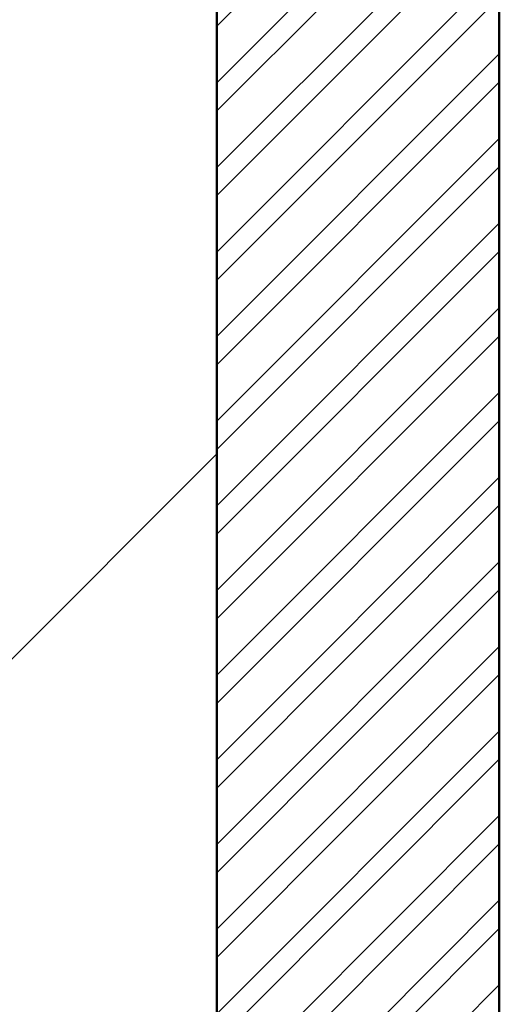
# Model space of a CAD drawing. Units: inches. Extents: x 3590 to 5167, y 65 to 1917.
# Tile 47 of 100: x 5065 to 5080, y 1418 to 1450. Entities that reach past the tile are written whole.
import ezdxf

# ---------------------------------------------------------------- set-up
doc = ezdxf.new("R2010")
doc.units = ezdxf.units.IN
for name, color, linetype, lineweight in [('A-FLOR-PATT', 8, 'Continuous', 13), ('A-WALL', 7, 'Continuous', 50), ('A-WALL-PATT', 251, 'Continuous', 13)]:
    doc.layers.add(name, color=color, linetype=linetype, lineweight=lineweight)

msp = doc.modelspace()

# ---------------------------------------------------------------- hatches: boundary and pattern name
at = {"layer": 'A-FLOR-PATT', "transparency": 33554687}
h = msp.add_hatch(dxfattribs=at)
h.set_pattern_fill('AR-HBONE', color=256, scale=0.2)
h.set_pattern_definition([(45, (-588.972, 0), (0, 28.73682), [60.96, -20.32]), (135, (-574.604, 14.368), (3e-15, 28.73682), [60.96, -20.32])])
h.paths.add_polyline_path([(5071.274, 1796.999), (4933.274, 1796.999), (4933.274, 1753.999), (4962.774, 1753.999, -0.414214), (4928.774, 1719.999), (4933.274, 1718.999), (4933.274, 1334.999), (5071.274, 1334.999)])
h.paths.add_polyline_path([(4951.78, 1521.077), (4951.715, 1521.04), (4951.563, 1520.895)], flags=16)
h.paths.add_polyline_path([(4952.267, 1521.376), (4952.198, 1521.371), (4952.198, 1521.356)], flags=0)
h.paths.add_polyline_path([(4967.051, 1529.728), (4965.231, 1528.694), (4963.411, 1527.714), (4961.756, 1526.851), (4963.589, 1527.449), (4964.036, 1527.478), (4962.975, 1527.249), (4961.76, 1526.852), (4959.792, 1525.834), (4958.005, 1524.895), (4956.24, 1523.93), (4954.504, 1522.919), (4954.129, 1522.682), (4953.361, 1521.997), (4953.366, 1521.998), (4953.605, 1522.064), (4955.106, 1522.761), (4956.921, 1523.434), (4958.678, 1523.915), (4960.358, 1524.2), (4961.945, 1524.286), (4964.171, 1524.108), (4965.958, 1523.309), (4963.863, 1522.976), (4965.187, 1522.499), (4963.366, 1522.497), (4961.545, 1522.487), (4959.764, 1522.461), (4958.304, 1522.419), (4957.974, 1522.388), (4956.307, 1522.232), (4954.718, 1522.071), (4953.251, 1521.899), (4953.525, 1521.623), (4954.331, 1521.379), (4956.243, 1521.23), (4958.039, 1520.93), (4959.684, 1520.483), (4961.16, 1519.896), (4963.107, 1518.8), (4964.393, 1517.325), (4962.973, 1517.726), (4964.558, 1516.661), (4965.407, 1515.708), (4963.507, 1516.322), (4961.68, 1517.005), (4959.935, 1517.745), (4958.282, 1518.528), (4956.732, 1519.343), (4955.295, 1520.175), (4954.672, 1520.572), (4954.513, 1520.627), (4955.658, 1519.318), (4956.703, 1517.982), (4957.644, 1516.647), (4958.485, 1515.334), (4959.55, 1513.524), (4960.438, 1511.769), (4958.841, 1513.62), (4957.452, 1515.325), (4955.819, 1517.459), (4956.665, 1515.448), (4957.111, 1513.923), (4957.447, 1511.714), (4957.076, 1509.793), (4956.538, 1511.11), (4955.992, 1512.569), (4955.444, 1514.125), (4954.898, 1515.735), (4954.357, 1517.356), (4953.824, 1518.943), (4953.305, 1520.452), (4953.065, 1521.116), (4952.971, 1521.146), (4952.949, 1521.086), (4952.73, 1520.199), (4953.37, 1518.024), (4953.757, 1516.373), (4954.051, 1514.765), (4954.264, 1513.221), (4954.471, 1511.131), (4954.497, 1510.402), (4954.409, 1511.76), (4954.264, 1513.221), (4954.051, 1514.765), (4953.757, 1516.373), (4953.37, 1518.024), (4952.877, 1519.698), (4952.716, 1520.141), (4952.533, 1519.059), (4952.374, 1517.789), (4952.219, 1516.312), (4952.046, 1514.6), (4951.833, 1512.626), (4951.557, 1510.363), (4951.203, 1512.168), (4950.852, 1514.339), (4950.985, 1516.376), (4951.66, 1518.286), (4952.593, 1520.481), (4952.357, 1521.13), (4951.855, 1520.328), (4950.839, 1518.908), (4949.777, 1517.587), (4948.916, 1516.617), (4948.111, 1515.256), (4947.089, 1513.554), (4945.889, 1511.615), (4946.326, 1513.402), (4946.562, 1514.249), (4945.528, 1513.327), (4944.581, 1512.531), (4946.018, 1514.508), (4947.204, 1516.048), (4947.893, 1517.313), (4949.307, 1518.764), (4950.414, 1519.767), (4950.451, 1519.806), (4952.267, 1521.376), (4951.645, 1521.493), (4950.404, 1521.18), (4948.044, 1520.359), (4946.119, 1519.452), (4944.572, 1518.475), (4943.35, 1517.443), (4941.997, 1515.92), (4941.661, 1515.275), (4942.813, 1516.99), (4944.572, 1518.475), (4946.119, 1519.452), (4948.044, 1520.359), (4950.404, 1521.18), (4951.645, 1521.493), (4949.647, 1521.868), (4948.6, 1521.756), (4947.126, 1521.57), (4945.42, 1521.348), (4943.45, 1521.105), (4941.183, 1520.856), (4942.86, 1521.613), (4943.873, 1522.03), (4942.952, 1521.909), (4941.41, 1521.485), (4939.543, 1520.67), (4938.968, 1520.226), (4940.733, 1521.299), (4942.952, 1521.909), (4943.702, 1522.008), (4945.894, 1522.7), (4947.565, 1522.714), (4948.921, 1522.566), (4951.131, 1522.183), (4950.971, 1522.297), (4948.129, 1523.006), (4946.035, 1523.707), (4944.232, 1524.521), (4942.707, 1525.461), (4941.444, 1526.537), (4940.43, 1527.761), (4939.649, 1529.143), (4941.421, 1528.122), (4943.147, 1527.132), (4944.841, 1526.175), (4946.514, 1525.25), (4948.179, 1524.359), (4948.365, 1524.263), (4946.475, 1526.045), (4945.181, 1527.54), (4944.19, 1529.033), (4943.496, 1530.54), (4943.278, 1531.36), (4942.498, 1531.919), (4943.114, 1531.762), (4942.959, 1533.659), (4944.14, 1531.989), (4944.612, 1531.323), (4946.202, 1530.463), (4947.486, 1529.509), (4948.79, 1528.226), (4950.368, 1526.237), (4949.485, 1528.155), (4948.851, 1530.123), (4948.491, 1532.041), (4948.381, 1533.918), (4948.501, 1535.76), (4948.827, 1537.573), (4949.418, 1535.565), (4949.957, 1533.569), (4950.464, 1531.586), (4950.961, 1529.617), (4951.391, 1527.954), (4951.724, 1530.687), (4952.201, 1532.58), (4952.889, 1534.33), (4953.77, 1535.951), (4954.827, 1537.46), (4954.521, 1535.39), (4954.273, 1533.937), (4955.58, 1535.663), (4956.748, 1536.739), (4956.159, 1534.78), (4955.589, 1532.873), (4955.043, 1531.006), (4954.525, 1529.166), (4954.038, 1527.341), (4953.638, 1525.733), (4953.611, 1525.586), (4953.398, 1524.166), (4953.382, 1524.009), (4954.07, 1525.476), (4954.912, 1527.022), (4956.136, 1528.894), (4957.847, 1530.577), (4959.376, 1531.54), (4958.256, 1530.104), (4957.143, 1528.663), (4956.066, 1527.243), (4955.056, 1525.871), (4954.141, 1524.571), (4953.352, 1523.372), (4953.311, 1523.303), (4953.273, 1522.925), (4953.261, 1522.382), (4954.103, 1523.373), (4954.63, 1524.284), (4955.961, 1526.358), (4957.23, 1528.13), (4958.421, 1529.609), (4960.037, 1531.368), (4961.374, 1532.375), (4962.101, 1532.77), (4961.07, 1531.061), (4959.987, 1529.438), (4958.869, 1527.908), (4958.15, 1527.007), (4959.803, 1528.003), (4961.589, 1528.793), (4963.391, 1529.328), (4965.211, 1529.632)], flags=16)
h.paths.add_polyline_path([(4962.944, 1523.182), (4961.107, 1523.422), (4960.392, 1523.362), (4962.35, 1523.331)], flags=0)
h.paths.add_polyline_path([(5049.541, 1584.551), (5049.476, 1584.515), (5049.325, 1584.37)], flags=16)
h.paths.add_polyline_path([(5050.028, 1584.851), (5049.959, 1584.845), (5049.959, 1584.83)], flags=0)
h.paths.add_polyline_path([(5042.333, 1581.949), (5043.88, 1582.926), (5045.806, 1583.833), (5048.165, 1584.654), (5049.406, 1584.967), (5047.408, 1585.342), (5046.361, 1585.231), (5044.888, 1585.044), (5043.181, 1584.822), (5041.211, 1584.579), (5038.944, 1584.33), (5040.622, 1585.087), (5041.634, 1585.504), (5040.713, 1585.383), (5039.171, 1584.959), (5037.304, 1584.144), (5036.729, 1583.7), (5038.494, 1584.773), (5040.713, 1585.383), (5041.463, 1585.482), (5043.655, 1586.174), (5045.326, 1586.188), (5046.682, 1586.04), (5048.893, 1585.657), (5048.732, 1585.771), (5045.891, 1586.48), (5043.796, 1587.181), (5041.994, 1587.996), (5040.468, 1588.935), (5039.205, 1590.011), (5038.191, 1591.235), (5037.41, 1592.617), (5039.182, 1591.596), (5040.909, 1590.607), (5042.602, 1589.649), (5044.275, 1588.724), (5045.94, 1587.833), (5046.126, 1587.738), (5044.237, 1589.519), (5042.942, 1591.015), (5041.952, 1592.508), (5041.257, 1594.014), (5041.039, 1594.834), (5040.26, 1595.393), (5040.875, 1595.237), (5040.721, 1597.133), (5041.901, 1595.463), (5042.373, 1594.798), (5043.963, 1593.938), (5045.247, 1592.983), (5046.552, 1591.701), (5048.129, 1589.712), (5047.247, 1591.63), (5046.613, 1593.597), (5046.252, 1595.515), (5046.142, 1597.392), (5046.262, 1599.234), (5046.588, 1601.047), (5047.179, 1599.039), (5047.718, 1597.043), (5048.225, 1595.06), (5048.722, 1593.091), (5049.152, 1591.429), (5049.485, 1594.161), (5049.962, 1596.054), (5050.65, 1597.804), (5051.532, 1599.425), (5052.589, 1600.934), (5052.283, 1598.864), (5052.034, 1597.411), (5053.341, 1599.137), (5054.509, 1600.213), (5053.92, 1598.254), (5053.35, 1596.348), (5052.805, 1594.48), (5052.286, 1592.64), (5051.799, 1590.815), (5051.4, 1589.207), (5051.373, 1589.06), (5051.159, 1587.64), (5051.143, 1587.483), (5051.831, 1588.95), (5052.673, 1590.496), (5053.898, 1592.368), (5055.608, 1594.051), (5057.137, 1595.014), (5056.017, 1593.578), (5054.904, 1592.137), (5053.828, 1590.717), (5052.817, 1589.345), (5051.902, 1588.046), (5051.113, 1586.846), (5051.072, 1586.777), (5051.034, 1586.399), (5051.022, 1585.856), (5051.864, 1586.847), (5052.391, 1587.758), (5053.723, 1589.832), (5054.991, 1591.604), (5056.182, 1593.083), (5057.798, 1594.842), (5059.135, 1595.849), (5059.863, 1596.244), (5058.831, 1594.535), (5057.749, 1592.912), (5056.63, 1591.382), (5055.912, 1590.482), (5057.564, 1591.477), (5059.35, 1592.267), (5061.152, 1592.802), (5062.972, 1593.106), (5064.812, 1593.203), (5062.992, 1592.169), (5061.172, 1591.188), (5059.518, 1590.325), (5061.35, 1590.924), (5061.797, 1590.952), (5060.737, 1590.723), (5059.521, 1590.326), (5057.553, 1589.308), (5055.766, 1588.369), (5054.002, 1587.404), (5052.265, 1586.393), (5051.891, 1586.156), (5051.122, 1585.471), (5051.127, 1585.472), (5051.366, 1585.538), (5052.867, 1586.235), (5054.682, 1586.908), (5056.439, 1587.389), (5058.12, 1587.675), (5059.706, 1587.76), (5061.933, 1587.583), (5063.719, 1586.783), (5061.624, 1586.45), (5062.949, 1585.973), (5061.127, 1585.971), (5059.307, 1585.961), (5057.525, 1585.935), (5056.065, 1585.893), (5055.735, 1585.862), (5054.068, 1585.707), (5052.479, 1585.546), (5051.012, 1585.373), (5051.286, 1585.097), (5052.092, 1584.853), (5054.004, 1584.704), (5055.8, 1584.404), (5057.446, 1583.958), (5058.921, 1583.37), (5060.868, 1582.274), (5062.154, 1580.799), (5060.734, 1581.2), (5062.32, 1580.135), (5063.168, 1579.182), (5061.269, 1579.796), (5059.441, 1580.479), (5057.696, 1581.219), (5056.043, 1582.003), (5054.493, 1582.817), (5053.057, 1583.649), (5052.433, 1584.047), (5052.274, 1584.101), (5053.42, 1582.793), (5054.464, 1581.457), (5055.405, 1580.121), (5056.247, 1578.809), (5057.311, 1576.998), (5058.199, 1575.244), (5056.602, 1577.094), (5055.213, 1578.799), (5053.58, 1580.933), (5054.427, 1578.922), (5054.872, 1577.397), (5055.208, 1575.189), (5054.838, 1573.267), (5054.299, 1574.584), (5053.754, 1576.043), (5053.206, 1577.599), (5052.659, 1579.209), (5052.118, 1580.83), (5051.585, 1582.417), (5051.066, 1583.927), (5050.826, 1584.59), (5050.733, 1584.62), (5050.711, 1584.561), (5050.491, 1583.673), (5051.131, 1581.498), (5051.518, 1579.847), (5051.813, 1578.24), (5052.026, 1576.695), (5052.233, 1574.605), (5052.258, 1573.876), (5052.17, 1575.234), (5052.026, 1576.695), (5051.813, 1578.24), (5051.518, 1579.847), (5051.131, 1581.498), (5050.638, 1583.172), (5050.477, 1583.615), (5050.294, 1582.533), (5050.136, 1581.263), (5049.981, 1579.786), (5049.807, 1578.074), (5049.594, 1576.1), (5049.318, 1573.837), (5048.965, 1575.642), (5048.613, 1577.813), (5048.747, 1579.85), (5049.421, 1581.76), (5050.354, 1583.955), (5050.118, 1584.604), (5049.616, 1583.802), (5048.6, 1582.382), (5047.538, 1581.061), (5046.677, 1580.091), (5045.872, 1578.73), (5044.85, 1577.028), (5043.651, 1575.089), (5044.087, 1576.877), (5044.324, 1577.723), (5043.289, 1576.801), (5042.342, 1576.005), (5043.779, 1577.982), (5044.966, 1579.522), (5045.655, 1580.787), (5047.068, 1582.239), (5048.175, 1583.241), (5048.213, 1583.28), (5050.028, 1584.851), (5049.406, 1584.967), (5048.165, 1584.654), (5045.806, 1583.833), (5043.88, 1582.926), (5042.333, 1581.949), (5041.111, 1580.917), (5039.758, 1579.394), (5039.423, 1578.749), (5040.575, 1580.464)], flags=16)
h.paths.add_polyline_path([(4954.799, 1533.12), (4954.262, 1532.079), (4953.831, 1530.935), (4953.505, 1529.636), (4953.283, 1528.133), (4953.167, 1526.376), (4953.156, 1524.315), (4953.277, 1521.236), (4952.802, 1521.842), (4951.557, 1521.998), (4950.976, 1521.961), (4952.661, 1521.941), (4952.802, 1521.842), (4953.152, 1523.593), (4953.167, 1526.376), (4953.283, 1528.133), (4953.609, 1530.346), (4954.456, 1532.592)], flags=0)
h.paths.add_polyline_path([(5050.563, 1585.316), (5049.318, 1585.472), (5048.737, 1585.435), (5050.422, 1585.415), (5050.563, 1585.316), (5050.914, 1587.067), (5050.928, 1589.851), (5051.045, 1591.607), (5051.371, 1593.82), (5052.217, 1596.066), (5052.56, 1596.594), (5052.024, 1595.554), (5051.592, 1594.409), (5051.266, 1593.11), (5051.045, 1591.607), (5050.928, 1589.851), (5050.918, 1587.789), (5051.038, 1584.71)], flags=0)
h.paths.add_polyline_path([(5058.153, 1586.836), (5060.111, 1586.805), (5060.705, 1586.656), (5058.868, 1586.896)], flags=0)
h.paths.add_polyline_path([(5049.541, 1430.936), (5049.476, 1430.9), (5049.325, 1430.755)], flags=16)
h.paths.add_polyline_path([(5050.028, 1431.236), (5049.959, 1431.231), (5049.959, 1431.215)], flags=0)
h.paths.add_polyline_path([(5046.588, 1447.432), (5047.179, 1445.425), (5047.718, 1443.429), (5048.225, 1441.446), (5048.722, 1439.476), (5049.152, 1437.814), (5049.485, 1440.546), (5049.962, 1442.439), (5050.65, 1444.189), (5051.532, 1445.811), (5052.589, 1447.319), (5052.283, 1445.249), (5052.034, 1443.796), (5053.341, 1445.522), (5054.509, 1446.598), (5053.92, 1444.64), (5053.35, 1442.733), (5052.805, 1440.865), (5052.286, 1439.025), (5051.799, 1437.201), (5051.4, 1435.592), (5051.373, 1435.445), (5051.159, 1434.025), (5051.143, 1433.868), (5051.831, 1435.335), (5052.673, 1436.881), (5053.898, 1438.753), (5055.608, 1440.436), (5057.137, 1441.4), (5056.017, 1439.963), (5054.904, 1438.522), (5053.828, 1437.102), (5052.817, 1435.73), (5051.902, 1434.431), (5051.113, 1433.231), (5051.072, 1433.162), (5051.034, 1432.784), (5051.022, 1432.242), (5051.864, 1433.232), (5052.391, 1434.143), (5053.723, 1436.217), (5054.991, 1437.989), (5056.182, 1439.468), (5057.798, 1441.227), (5059.135, 1442.235), (5059.863, 1442.629), (5058.831, 1440.921), (5057.749, 1439.298), (5056.63, 1437.767), (5055.912, 1436.867), (5057.564, 1437.863), (5059.35, 1438.652), (5061.152, 1439.187), (5062.972, 1439.491), (5064.812, 1439.588), (5062.992, 1438.554), (5061.172, 1437.573), (5059.518, 1436.71), (5061.35, 1437.309), (5061.797, 1437.337), (5060.737, 1437.108), (5059.521, 1436.711), (5057.553, 1435.693), (5055.766, 1434.754), (5054.002, 1433.789), (5052.265, 1432.778), (5051.891, 1432.541), (5051.122, 1431.856), (5051.127, 1431.857), (5051.366, 1431.923), (5052.867, 1432.62), (5054.682, 1433.293), (5056.439, 1433.775), (5058.12, 1434.06), (5059.706, 1434.145), (5061.933, 1433.968), (5063.719, 1433.168), (5061.624, 1432.835), (5062.949, 1432.358), (5061.127, 1432.357), (5059.307, 1432.346), (5057.525, 1432.32), (5056.065, 1432.278), (5055.735, 1432.248), (5054.068, 1432.092), (5052.479, 1431.931), (5051.012, 1431.759), (5051.286, 1431.482), (5052.092, 1431.238), (5054.004, 1431.089), (5055.8, 1430.789), (5057.446, 1430.343), (5058.921, 1429.755), (5060.868, 1428.66), (5062.154, 1427.185), (5060.734, 1427.585), (5062.32, 1426.52), (5063.168, 1425.567), (5061.269, 1426.181), (5059.441, 1426.865), (5057.696, 1427.604), (5056.043, 1428.388), (5054.493, 1429.202), (5053.057, 1430.034), (5052.433, 1430.432), (5052.274, 1430.487), (5053.42, 1429.178), (5054.464, 1427.842), (5055.405, 1426.506), (5056.247, 1425.194), (5057.311, 1423.383), (5058.199, 1421.629), (5056.602, 1423.479), (5055.213, 1425.184), (5053.58, 1427.318), (5054.427, 1425.307), (5054.872, 1423.782), (5055.208, 1421.574), (5054.838, 1419.652), (5054.299, 1420.97), (5053.754, 1422.428), (5053.206, 1423.984), (5052.659, 1425.595), (5052.118, 1427.215), (5051.585, 1428.802), (5051.066, 1430.312), (5050.826, 1430.975), (5050.733, 1431.005), (5050.711, 1430.946), (5050.491, 1430.058), (5051.131, 1427.883), (5051.518, 1426.232), (5051.813, 1424.625), (5052.026, 1423.081), (5052.233, 1420.991), (5052.258, 1420.261), (5052.17, 1421.619), (5052.026, 1423.081), (5051.813, 1424.625), (5051.518, 1426.232), (5051.131, 1427.883), (5050.638, 1429.558), (5050.477, 1430.001), (5050.294, 1428.918), (5050.136, 1427.648), (5049.981, 1426.171), (5049.807, 1424.459), (5049.594, 1422.485), (5049.318, 1420.222), (5048.965, 1422.028), (5048.613, 1424.199), (5048.747, 1426.235), (5049.421, 1428.146), (5050.354, 1430.34), (5050.118, 1430.989), (5049.616, 1430.187), (5048.6, 1428.768), (5047.538, 1427.446), (5046.677, 1426.477), (5045.872, 1425.116), (5044.85, 1423.413), (5043.651, 1421.474), (5044.087, 1423.262), (5044.324, 1424.109), (5043.289, 1423.186), (5042.342, 1422.391), (5043.779, 1424.368), (5044.966, 1425.907), (5045.655, 1427.173), (5047.068, 1428.624), (5048.175, 1429.627), (5048.213, 1429.666), (5050.028, 1431.236), (5049.406, 1431.353), (5048.165, 1431.039), (5045.806, 1430.218), (5043.88, 1429.311), (5042.333, 1428.334), (5041.111, 1427.302), (5039.758, 1425.779), (5039.423, 1425.134), (5040.575, 1426.849), (5042.333, 1428.334), (5043.88, 1429.311), (5045.806, 1430.218), (5048.165, 1431.039), (5049.406, 1431.353), (5047.408, 1431.727), (5046.361, 1431.616), (5044.888, 1431.429), (5043.181, 1431.207), (5041.211, 1430.964), (5038.944, 1430.715), (5040.622, 1431.472), (5041.634, 1431.89), (5040.713, 1431.769), (5039.171, 1431.345), (5037.304, 1430.53), (5036.729, 1430.085), (5038.494, 1431.158), (5040.713, 1431.769), (5041.463, 1431.867), (5043.655, 1432.559), (5045.326, 1432.573), (5046.682, 1432.425), (5048.893, 1432.042), (5048.732, 1432.156), (5045.891, 1432.865), (5043.796, 1433.566), (5041.994, 1434.381), (5040.468, 1435.321), (5039.205, 1436.396), (5038.191, 1437.62), (5037.41, 1439.002), (5039.182, 1437.982), (5040.909, 1436.992), (5042.602, 1436.034), (5044.275, 1435.109), (5045.94, 1434.218), (5046.126, 1434.123), (5044.237, 1435.904), (5042.942, 1437.4), (5041.952, 1438.893), (5041.257, 1440.399), (5041.039, 1441.219), (5040.26, 1441.778), (5040.875, 1441.622), (5040.721, 1443.518), (5041.901, 1441.848), (5042.373, 1441.183), (5043.963, 1440.323), (5045.247, 1439.369), (5046.552, 1438.086), (5048.129, 1436.097), (5047.247, 1438.015), (5046.613, 1439.982), (5046.252, 1441.901), (5046.142, 1443.778), (5046.262, 1445.619)], flags=16)
h.paths.add_polyline_path([(5052.382, 1444.255), (5051.623, 1442.78), (5052.024, 1441.939), (5052.56, 1442.98)], flags=0)
h.paths.add_polyline_path([(5050.563, 1431.701), (5049.318, 1431.857), (5048.737, 1431.821), (5050.422, 1431.8)], flags=0)
h.paths.add_polyline_path([(5058.153, 1433.221), (5060.111, 1433.19), (5060.705, 1433.041), (5058.868, 1433.281)], flags=0)
h.paths.add_polyline_path([(5049.541, 1352.285), (5049.476, 1352.249), (5049.325, 1352.104)], flags=16)
h.paths.add_polyline_path([(5050.028, 1352.585), (5049.959, 1352.58), (5049.959, 1352.564)], flags=0)
h.paths.add_polyline_path([(5046.588, 1368.781), (5047.179, 1366.774), (5047.718, 1364.778), (5048.225, 1362.795), (5048.722, 1360.825), (5049.152, 1359.163), (5049.485, 1361.896), (5049.962, 1363.789), (5050.65, 1365.538), (5051.532, 1367.16), (5052.589, 1368.669), (5052.283, 1366.598), (5052.034, 1365.145), (5053.341, 1366.871), (5054.509, 1367.947), (5053.92, 1365.989), (5053.35, 1364.082), (5052.805, 1362.214), (5052.286, 1360.374), (5051.799, 1358.55), (5051.4, 1356.942), (5051.373, 1356.794), (5051.159, 1355.374), (5051.143, 1355.218), (5051.831, 1356.684), (5052.673, 1358.23), (5053.898, 1360.102), (5055.608, 1361.786), (5057.137, 1362.749), (5056.017, 1361.313), (5054.904, 1359.872), (5053.828, 1358.452), (5052.817, 1357.079), (5051.902, 1355.78), (5051.113, 1354.581), (5051.072, 1354.512), (5051.034, 1354.133), (5051.022, 1353.591), (5051.864, 1354.581), (5052.391, 1355.492), (5053.723, 1357.566), (5054.991, 1359.338), (5056.182, 1360.817), (5057.798, 1362.577), (5059.135, 1363.584), (5059.863, 1363.979), (5058.831, 1362.27), (5057.749, 1360.647), (5056.63, 1359.117), (5055.912, 1358.216), (5057.564, 1359.212), (5059.35, 1360.001), (5061.152, 1360.536), (5062.972, 1360.841), (5064.812, 1360.937), (5062.992, 1359.903), (5061.172, 1358.923), (5059.518, 1358.059), (5061.35, 1358.658), (5061.797, 1358.687), (5060.737, 1358.458), (5059.521, 1358.061), (5057.553, 1357.043), (5055.766, 1356.103), (5054.002, 1355.138), (5052.265, 1354.127), (5051.891, 1353.89), (5051.122, 1353.206), (5051.127, 1353.206), (5051.366, 1353.272), (5052.867, 1353.969), (5054.682, 1354.643), (5056.439, 1355.124), (5058.12, 1355.409), (5059.706, 1355.495), (5061.933, 1355.317), (5063.719, 1354.518), (5061.624, 1354.184), (5062.949, 1353.708), (5061.127, 1353.706), (5059.307, 1353.695), (5057.525, 1353.669), (5056.065, 1353.627), (5055.735, 1353.597), (5054.068, 1353.441), (5052.479, 1353.28), (5051.012, 1353.108), (5051.286, 1352.831), (5052.092, 1352.587), (5054.004, 1352.439), (5055.8, 1352.138), (5057.446, 1351.692), (5058.921, 1351.104), (5060.868, 1350.009), (5062.154, 1348.534), (5060.734, 1348.935), (5062.32, 1347.869), (5063.168, 1346.916), (5061.269, 1347.53), (5059.441, 1348.214), (5057.696, 1348.954), (5056.043, 1349.737), (5054.493, 1350.551), (5053.057, 1351.383), (5052.433, 1351.781), (5052.274, 1351.836), (5053.42, 1350.527), (5054.464, 1349.191), (5055.405, 1347.855), (5056.247, 1346.543), (5057.311, 1344.733), (5058.199, 1342.978), (5056.602, 1344.828), (5055.213, 1346.534), (5053.58, 1348.667), (5054.427, 1346.656), (5054.872, 1345.132), (5055.208, 1342.923), (5054.838, 1341.002), (5054.299, 1342.319), (5053.754, 1343.778), (5053.206, 1345.334), (5052.659, 1346.944), (5052.118, 1348.564), (5051.585, 1350.151), (5051.066, 1351.661), (5050.826, 1352.324), (5050.733, 1352.355), (5050.711, 1352.295), (5050.491, 1351.408), (5051.131, 1349.232), (5051.518, 1347.581), (5051.813, 1345.974), (5052.026, 1344.43), (5052.233, 1342.34), (5052.258, 1341.61), (5052.17, 1342.969), (5052.026, 1344.43), (5051.813, 1345.974), (5051.518, 1347.581), (5051.131, 1349.232), (5050.638, 1350.907), (5050.477, 1351.35), (5050.294, 1350.267), (5050.136, 1348.997), (5049.981, 1347.52), (5049.807, 1345.809), (5049.594, 1343.835), (5049.318, 1341.571), (5048.965, 1343.377), (5048.613, 1345.548), (5048.747, 1347.585), (5049.421, 1349.495), (5050.354, 1351.689), (5050.118, 1352.339), (5049.616, 1351.536), (5048.6, 1350.117), (5047.538, 1348.795), (5046.677, 1347.826), (5045.872, 1346.465), (5044.85, 1344.763), (5043.651, 1342.824), (5044.087, 1344.611), (5044.324, 1345.458), (5043.289, 1344.535), (5042.342, 1343.74), (5043.779, 1345.717), (5044.966, 1347.256), (5045.655, 1348.522), (5047.068, 1349.973), (5048.175, 1350.976), (5048.213, 1351.015), (5050.028, 1352.585), (5049.406, 1352.702), (5048.165, 1352.388), (5045.806, 1351.567), (5043.88, 1350.661), (5042.333, 1349.683), (5041.111, 1348.651), (5039.758, 1347.128), (5039.423, 1346.483), (5040.575, 1348.198), (5042.333, 1349.683), (5043.88, 1350.661), (5045.806, 1351.567), (5048.165, 1352.388), (5049.406, 1352.702), (5047.408, 1353.076), (5046.361, 1352.965), (5044.888, 1352.779), (5043.181, 1352.556), (5041.211, 1352.313), (5038.944, 1352.065), (5040.622, 1352.821), (5041.634, 1353.239), (5040.713, 1353.118), (5039.171, 1352.694), (5037.304, 1351.879), (5036.729, 1351.434), (5038.494, 1352.508), (5040.713, 1353.118), (5041.463, 1353.216), (5043.655, 1353.909), (5045.326, 1353.923), (5046.682, 1353.774), (5048.893, 1353.391), (5048.732, 1353.506), (5045.891, 1354.214), (5043.796, 1354.915), (5041.994, 1355.73), (5040.468, 1356.67), (5039.205, 1357.746), (5038.191, 1358.969), (5037.41, 1360.352), (5039.182, 1359.331), (5040.909, 1358.341), (5042.602, 1357.383), (5044.275, 1356.458), (5045.94, 1355.567), (5046.126, 1355.472), (5044.237, 1357.253), (5042.942, 1358.749), (5041.952, 1360.242), (5041.257, 1361.748), (5041.039, 1362.568), (5040.26, 1363.128), (5040.875, 1362.971), (5040.721, 1364.867), (5041.901, 1363.197), (5042.373, 1362.532), (5043.963, 1361.672), (5045.247, 1360.718), (5046.552, 1359.435), (5048.129, 1357.446), (5047.247, 1359.364), (5046.613, 1361.331), (5046.252, 1363.25), (5046.142, 1365.127), (5046.262, 1366.969)], flags=16)
h.paths.add_polyline_path([(5052.382, 1365.604), (5051.623, 1364.129), (5052.024, 1363.288), (5052.56, 1364.329)], flags=0)
h.paths.add_polyline_path([(4951.78, 1698.041), (4951.715, 1698.005), (4951.563, 1697.859)], flags=16)
h.paths.add_polyline_path([(4952.267, 1698.341), (4952.198, 1698.335), (4952.198, 1698.32)], flags=0)
h.paths.add_polyline_path([(4957.076, 1686.757), (4956.538, 1688.074), (4955.992, 1689.533), (4955.444, 1691.089), (4954.898, 1692.699), (4954.357, 1694.32), (4953.824, 1695.907), (4953.305, 1697.417), (4953.065, 1698.08), (4952.971, 1698.11), (4952.949, 1698.051), (4952.73, 1697.163), (4953.37, 1694.988), (4953.757, 1693.337), (4954.051, 1691.729), (4954.264, 1690.185), (4954.471, 1688.095), (4954.497, 1687.366), (4954.409, 1688.724), (4954.264, 1690.185), (4954.051, 1691.729), (4953.757, 1693.337), (4953.37, 1694.988), (4952.877, 1696.662), (4952.716, 1697.105), (4952.533, 1696.023), (4952.374, 1694.753), (4952.219, 1693.276), (4952.046, 1691.564), (4951.833, 1689.59), (4951.557, 1687.327), (4951.203, 1689.132), (4950.852, 1691.303), (4950.985, 1693.34), (4951.66, 1695.25), (4952.593, 1697.445), (4952.357, 1698.094), (4951.855, 1697.292), (4950.839, 1695.872), (4949.777, 1694.551), (4948.916, 1693.581), (4948.111, 1692.22), (4947.089, 1690.518), (4945.889, 1688.579), (4946.326, 1690.366), (4946.562, 1691.213), (4945.528, 1690.291), (4944.581, 1689.495), (4946.018, 1691.472), (4947.204, 1693.012), (4947.893, 1694.277), (4949.307, 1695.729), (4950.414, 1696.731), (4950.451, 1696.77), (4952.267, 1698.341), (4951.645, 1698.457), (4950.404, 1698.144), (4948.044, 1697.323), (4946.119, 1696.416), (4944.572, 1695.439), (4943.35, 1694.407), (4941.997, 1692.884), (4941.661, 1692.239), (4942.813, 1693.954), (4944.572, 1695.439), (4946.119, 1696.416), (4948.044, 1697.323), (4950.404, 1698.144), (4951.645, 1698.457), (4949.647, 1698.832), (4948.6, 1698.72), (4947.126, 1698.534), (4945.42, 1698.312), (4943.45, 1698.069), (4941.183, 1697.82), (4942.86, 1698.577), (4943.873, 1698.994), (4942.952, 1698.873), (4941.41, 1698.449), (4939.543, 1697.634), (4938.968, 1697.19), (4940.733, 1698.263), (4942.952, 1698.873), (4943.702, 1698.972), (4945.894, 1699.664), (4947.565, 1699.678), (4948.921, 1699.53), (4951.131, 1699.147), (4950.971, 1699.261), (4948.129, 1699.97), (4946.035, 1700.671), (4944.232, 1701.486), (4942.707, 1702.425), (4941.444, 1703.501), (4940.43, 1704.725), (4939.649, 1706.107), (4941.421, 1705.086), (4943.147, 1704.097), (4944.841, 1703.139), (4946.514, 1702.214), (4948.179, 1701.323), (4948.365, 1701.227), (4946.475, 1703.009), (4945.181, 1704.505), (4944.19, 1705.997), (4943.496, 1707.504), (4943.278, 1708.324), (4942.498, 1708.883), (4943.114, 1708.727), (4942.959, 1710.623), (4944.14, 1708.953), (4944.612, 1708.287), (4946.202, 1707.428), (4947.486, 1706.473), (4948.79, 1705.191), (4950.368, 1703.202), (4949.485, 1705.12), (4948.851, 1707.087), (4948.491, 1709.005), (4948.381, 1710.882), (4948.501, 1712.724), (4948.827, 1714.537), (4949.418, 1712.529), (4949.957, 1710.533), (4950.464, 1708.55), (4950.961, 1706.581), (4951.391, 1704.919), (4951.724, 1707.651), (4952.201, 1709.544), (4952.889, 1711.294), (4953.77, 1712.915), (4954.827, 1714.424), (4954.521, 1712.354), (4954.273, 1710.901), (4955.58, 1712.627), (4956.748, 1713.703), (4956.159, 1711.744), (4955.589, 1709.837), (4955.043, 1707.97), (4954.525, 1706.13), (4954.038, 1704.305), (4953.638, 1702.697), (4953.611, 1702.55), (4953.398, 1701.13), (4953.382, 1700.973), (4954.07, 1702.44), (4954.912, 1703.986), (4956.136, 1705.858), (4957.847, 1707.541), (4959.376, 1708.504), (4958.256, 1707.068), (4957.143, 1705.627), (4956.066, 1704.207), (4955.056, 1702.835), (4954.141, 1701.536), (4953.352, 1700.336), (4953.311, 1700.267), (4953.273, 1699.889), (4953.261, 1699.346), (4954.103, 1700.337), (4954.63, 1701.248), (4955.961, 1703.322), (4957.23, 1705.094), (4958.421, 1706.573), (4960.037, 1708.332), (4961.374, 1709.339), (4962.101, 1709.734), (4961.07, 1708.025), (4959.987, 1706.402), (4958.869, 1704.872), (4958.15, 1703.972), (4959.803, 1704.967), (4961.589, 1705.757), (4963.391, 1706.292), (4965.211, 1706.596), (4967.051, 1706.692), (4965.231, 1705.659), (4963.411, 1704.678), (4961.756, 1703.815), (4963.589, 1704.413), (4964.036, 1704.442), (4962.975, 1704.213), (4961.76, 1703.816), (4959.792, 1702.798), (4958.005, 1701.859), (4956.24, 1700.894), (4954.504, 1699.883), (4954.129, 1699.646), (4953.361, 1698.961), (4953.366, 1698.962), (4953.605, 1699.028), (4955.106, 1699.725), (4956.921, 1700.398), (4958.678, 1700.879), (4960.358, 1701.164), (4961.945, 1701.25), (4964.171, 1701.073), (4965.958, 1700.273), (4963.863, 1699.94), (4965.187, 1699.463), (4963.366, 1699.461), (4961.545, 1699.451), (4959.764, 1699.425), (4958.304, 1699.383), (4957.974, 1699.352), (4956.307, 1699.197), (4954.718, 1699.036), (4953.251, 1698.863), (4953.525, 1698.587), (4954.331, 1698.343), (4956.243, 1698.194), (4958.039, 1697.894), (4959.684, 1697.447), (4961.16, 1696.86), (4963.107, 1695.764), (4964.393, 1694.289), (4962.973, 1694.69), (4964.558, 1693.625), (4965.407, 1692.672), (4963.507, 1693.286), (4961.68, 1693.969), (4959.935, 1694.709), (4958.282, 1695.492), (4956.732, 1696.307), (4955.295, 1697.139), (4954.672, 1697.536), (4954.513, 1697.591), (4955.658, 1696.282), (4956.703, 1694.946), (4957.644, 1693.611), (4958.485, 1692.298), (4959.55, 1690.488), (4960.438, 1688.733), (4958.841, 1690.584), (4957.452, 1692.289), (4955.819, 1694.423), (4956.665, 1692.412), (4957.111, 1690.887), (4957.447, 1688.678)], flags=16)
h.paths.add_polyline_path([(5050.563, 1353.05), (5049.318, 1353.207), (5048.737, 1353.17), (5050.422, 1353.15)], flags=0)
h.paths.add_polyline_path([(4951.78, 1351.486), (4951.715, 1351.45), (4951.563, 1351.305)], flags=16)
h.paths.add_polyline_path([(4952.267, 1351.786), (4952.198, 1351.78), (4952.198, 1351.765)], flags=0)
h.paths.add_polyline_path([(4954.827, 1367.869), (4954.521, 1365.799), (4954.273, 1364.346), (4955.58, 1366.072), (4956.748, 1367.148), (4956.159, 1365.19), (4955.589, 1363.283), (4955.043, 1361.415), (4954.525, 1359.575), (4954.038, 1357.751), (4953.638, 1356.142), (4953.611, 1355.995), (4953.398, 1354.575), (4953.382, 1354.418), (4954.07, 1355.885), (4954.912, 1357.431), (4956.136, 1359.303), (4957.847, 1360.986), (4959.376, 1361.95), (4958.256, 1360.513), (4957.143, 1359.072), (4956.066, 1357.652), (4955.056, 1356.28), (4954.141, 1354.981), (4953.352, 1353.781), (4953.311, 1353.712), (4953.273, 1353.334), (4953.261, 1352.792), (4954.103, 1353.782), (4954.63, 1354.693), (4955.961, 1356.767), (4957.23, 1358.539), (4958.421, 1360.018), (4960.037, 1361.777), (4961.374, 1362.785), (4962.101, 1363.179), (4961.07, 1361.471), (4959.987, 1359.848), (4958.869, 1358.317), (4958.15, 1357.417), (4959.803, 1358.413), (4961.589, 1359.202), (4963.391, 1359.737), (4965.211, 1360.041), (4967.051, 1360.138), (4965.231, 1359.104), (4963.411, 1358.123), (4961.756, 1357.26), (4963.589, 1357.859), (4964.036, 1357.887), (4962.975, 1357.658), (4961.76, 1357.261), (4959.792, 1356.243), (4958.005, 1355.304), (4956.24, 1354.339), (4954.504, 1353.328), (4954.129, 1353.091), (4953.361, 1352.406), (4953.366, 1352.407), (4953.605, 1352.473), (4955.106, 1353.17), (4956.921, 1353.843), (4958.678, 1354.325), (4960.358, 1354.61), (4961.945, 1354.695), (4964.171, 1354.518), (4965.958, 1353.718), (4963.863, 1353.385), (4965.187, 1352.908), (4963.366, 1352.907), (4961.545, 1352.896), (4959.764, 1352.87), (4958.304, 1352.828), (4957.974, 1352.798), (4956.307, 1352.642), (4954.718, 1352.481), (4953.251, 1352.309), (4953.525, 1352.032), (4954.331, 1351.788), (4956.243, 1351.639), (4958.039, 1351.339), (4959.684, 1350.893), (4961.16, 1350.305), (4963.107, 1349.21), (4964.393, 1347.735), (4962.973, 1348.135), (4964.558, 1347.07), (4965.407, 1346.117), (4963.507, 1346.731), (4961.68, 1347.414), (4959.935, 1348.154), (4958.282, 1348.938), (4956.732, 1349.752), (4955.295, 1350.584), (4954.672, 1350.982), (4954.513, 1351.036), (4955.658, 1349.728), (4956.703, 1348.392), (4957.644, 1347.056), (4958.485, 1345.744), (4959.55, 1343.933), (4960.438, 1342.179), (4958.841, 1344.029), (4957.452, 1345.734), (4955.819, 1347.868), (4956.665, 1345.857), (4957.111, 1344.332), (4957.447, 1342.124), (4957.076, 1340.202), (4956.538, 1341.52), (4955.992, 1342.978), (4955.444, 1344.534), (4954.898, 1346.145), (4954.357, 1347.765), (4953.824, 1349.352), (4953.305, 1350.862), (4953.065, 1351.525), (4952.971, 1351.555), (4952.949, 1351.496), (4952.73, 1350.608), (4953.37, 1348.433), (4953.757, 1346.782), (4954.051, 1345.175), (4954.264, 1343.631), (4954.471, 1341.541), (4954.497, 1340.811), (4954.409, 1342.169), (4954.264, 1343.631), (4954.051, 1345.175), (4953.757, 1346.782), (4953.37, 1348.433), (4952.877, 1350.108), (4952.716, 1350.551), (4952.533, 1349.468), (4952.374, 1348.198), (4952.219, 1346.721), (4952.046, 1345.009), (4951.833, 1343.035), (4951.557, 1340.772), (4951.203, 1342.578), (4950.852, 1344.749), (4950.985, 1346.785), (4951.66, 1348.696), (4952.593, 1350.89), (4952.357, 1351.539), (4951.855, 1350.737), (4950.839, 1349.318), (4949.777, 1347.996), (4948.916, 1347.027), (4948.111, 1345.665), (4947.089, 1343.963), (4945.889, 1342.024), (4946.326, 1343.812), (4946.562, 1344.659), (4945.528, 1343.736), (4944.581, 1342.941), (4946.018, 1344.918), (4947.204, 1346.457), (4947.893, 1347.723), (4949.307, 1349.174), (4950.414, 1350.177), (4950.451, 1350.216), (4952.267, 1351.786), (4951.645, 1351.903), (4950.404, 1351.589), (4948.044, 1350.768), (4946.119, 1349.861), (4944.572, 1348.884), (4943.35, 1347.852), (4941.997, 1346.329), (4941.661, 1345.684), (4942.813, 1347.399), (4944.572, 1348.884), (4946.119, 1349.861), (4948.044, 1350.768), (4950.404, 1351.589), (4951.645, 1351.903), (4949.647, 1352.277), (4948.6, 1352.166), (4947.126, 1351.979), (4945.42, 1351.757), (4943.45, 1351.514), (4941.183, 1351.265), (4942.86, 1352.022), (4943.873, 1352.44), (4942.952, 1352.319), (4941.41, 1351.895), (4939.543, 1351.08), (4938.968, 1350.635), (4940.733, 1351.708), (4942.952, 1352.319), (4943.702, 1352.417), (4945.894, 1353.109), (4947.565, 1353.123), (4948.921, 1352.975), (4951.131, 1352.592), (4950.971, 1352.706), (4948.129, 1353.415), (4946.035, 1354.116), (4944.232, 1354.931), (4942.707, 1355.871), (4941.444, 1356.946), (4940.43, 1358.17), (4939.649, 1359.552), (4941.421, 1358.532), (4943.147, 1357.542), (4944.841, 1356.584), (4946.514, 1355.659), (4948.179, 1354.768), (4948.365, 1354.673), (4946.475, 1356.454), (4945.181, 1357.95), (4944.19, 1359.443), (4943.496, 1360.949), (4943.278, 1361.769), (4942.498, 1362.328), (4943.114, 1362.172), (4942.959, 1364.068), (4944.14, 1362.398), (4944.612, 1361.733), (4946.202, 1360.873), (4947.486, 1359.919), (4948.79, 1358.636), (4950.368, 1356.647), (4949.485, 1358.565), (4948.851, 1360.532), (4948.491, 1362.451), (4948.381, 1364.328), (4948.501, 1366.169), (4948.827, 1367.982), (4949.418, 1365.975), (4949.957, 1363.979), (4950.464, 1361.995), (4950.961, 1360.026), (4951.391, 1358.364), (4951.724, 1361.096), (4952.201, 1362.989), (4952.889, 1364.739), (4953.77, 1366.361)], flags=16)
h.paths.add_polyline_path([(4954.799, 1363.53), (4954.262, 1362.489), (4953.831, 1361.344), (4953.505, 1360.045), (4953.283, 1358.543), (4953.167, 1356.786), (4953.156, 1354.724), (4953.277, 1351.646), (4952.802, 1352.251), (4951.557, 1352.407), (4950.976, 1352.371), (4952.661, 1352.35), (4952.802, 1352.251), (4953.152, 1354.002), (4953.167, 1356.786), (4953.283, 1358.543), (4953.609, 1360.755), (4954.456, 1363.001)], flags=0)
h.paths.add_polyline_path([(4952.802, 1698.806), (4951.557, 1698.962), (4950.976, 1698.925), (4952.661, 1698.905), (4952.802, 1698.806), (4953.152, 1700.557), (4953.167, 1703.34), (4953.283, 1705.097), (4953.609, 1707.31), (4954.456, 1709.556), (4954.799, 1710.084), (4954.262, 1709.043), (4953.831, 1707.899), (4953.505, 1706.6), (4953.283, 1705.097), (4953.167, 1703.34), (4953.156, 1701.279), (4953.277, 1698.2)], flags=0)
h.paths.add_polyline_path([(4962.944, 1700.146), (4961.107, 1700.386), (4960.392, 1700.326), (4962.35, 1700.295)], flags=0)
h.paths.add_polyline_path([(5058.153, 1354.57), (5060.111, 1354.539), (5060.705, 1354.391), (5058.868, 1354.631)], flags=0)
h.paths.add_polyline_path([(4962.944, 1353.591), (4961.107, 1353.831), (4960.392, 1353.771), (4962.35, 1353.74)], flags=0)
h.paths.add_polyline_path([(5049.541, 1778.72), (5049.476, 1778.684), (5049.325, 1778.539)], flags=16)
h.paths.add_polyline_path([(5050.028, 1779.02), (5049.959, 1779.014), (5049.959, 1778.999)], flags=0)
h.paths.add_polyline_path([(5052.258, 1768.045), (5052.17, 1769.403), (5052.026, 1770.864), (5051.813, 1772.409), (5051.518, 1774.016), (5051.131, 1775.667), (5050.638, 1777.341), (5050.477, 1777.784), (5050.294, 1776.702), (5050.136, 1775.432), (5049.981, 1773.955), (5049.807, 1772.243), (5049.594, 1770.269), (5049.318, 1768.006), (5048.965, 1769.811), (5048.613, 1771.982), (5048.747, 1774.019), (5049.421, 1775.929), (5050.354, 1778.124), (5050.118, 1778.773), (5049.616, 1777.971), (5048.6, 1776.551), (5047.538, 1775.23), (5046.677, 1774.26), (5045.872, 1772.899), (5044.85, 1771.197), (5043.651, 1769.258), (5044.087, 1771.046), (5044.324, 1771.892), (5043.289, 1770.97), (5042.342, 1770.174), (5043.779, 1772.151), (5044.966, 1773.691), (5045.655, 1774.956), (5047.068, 1776.408), (5048.175, 1777.41), (5048.213, 1777.449), (5050.028, 1779.02), (5049.406, 1779.136), (5048.165, 1778.823), (5045.806, 1778.002), (5043.88, 1777.095), (5042.333, 1776.118), (5041.111, 1775.086), (5039.758, 1773.563), (5039.423, 1772.918), (5040.575, 1774.633), (5042.333, 1776.118), (5043.88, 1777.095), (5045.806, 1778.002), (5048.165, 1778.823), (5049.406, 1779.136), (5047.408, 1779.511), (5046.361, 1779.4), (5044.888, 1779.213), (5043.181, 1778.991), (5041.211, 1778.748), (5038.944, 1778.499), (5040.622, 1779.256), (5041.634, 1779.673), (5040.713, 1779.552), (5039.171, 1779.128), (5037.304, 1778.313), (5036.729, 1777.869), (5038.494, 1778.942), (5040.713, 1779.552), (5041.463, 1779.651), (5043.655, 1780.343), (5045.326, 1780.357), (5046.682, 1780.209), (5048.893, 1779.826), (5048.732, 1779.94), (5045.891, 1780.649), (5043.796, 1781.35), (5041.994, 1782.165), (5040.468, 1783.104), (5039.205, 1784.18), (5038.191, 1785.404), (5037.41, 1786.786), (5039.182, 1785.765), (5040.909, 1784.776), (5042.602, 1783.818), (5044.275, 1782.893), (5045.94, 1782.002), (5046.126, 1781.907), (5044.237, 1783.688), (5042.942, 1785.184), (5041.952, 1786.677), (5041.257, 1788.183), (5041.039, 1789.003), (5040.26, 1789.562), (5040.875, 1789.406), (5040.721, 1791.302), (5041.901, 1789.632), (5042.373, 1788.967), (5043.963, 1788.107), (5045.247, 1787.152), (5046.552, 1785.87), (5048.129, 1783.881), (5047.247, 1785.799), (5046.613, 1787.766), (5046.252, 1789.684), (5046.142, 1791.561), (5046.262, 1793.403), (5046.588, 1795.216), (5047.179, 1793.208), (5047.718, 1791.213), (5048.225, 1789.229), (5048.722, 1787.26), (5049.152, 1785.598), (5049.485, 1788.33), (5049.962, 1790.223), (5050.65, 1791.973), (5051.532, 1793.594), (5052.589, 1795.103), (5052.283, 1793.033), (5052.034, 1791.58), (5053.341, 1793.306), (5054.509, 1794.382), (5053.92, 1792.423), (5053.35, 1790.517), (5052.805, 1788.649), (5052.286, 1786.809), (5051.799, 1784.984), (5051.4, 1783.376), (5051.373, 1783.229), (5051.159, 1781.809), (5051.143, 1781.652), (5051.831, 1783.119), (5052.673, 1784.665), (5053.898, 1786.537), (5055.608, 1788.22), (5057.137, 1789.183), (5056.017, 1787.747), (5054.904, 1786.306), (5053.828, 1784.886), (5052.817, 1783.514), (5051.902, 1782.215), (5051.113, 1781.015), (5051.072, 1780.946), (5051.034, 1780.568), (5051.022, 1780.025), (5051.864, 1781.016), (5052.391, 1781.927), (5053.723, 1784.001), (5054.991, 1785.773), (5056.182, 1787.252), (5057.798, 1789.011), (5059.135, 1790.018), (5059.863, 1790.413), (5058.831, 1788.704), (5057.749, 1787.081), (5056.63, 1785.551), (5055.912, 1784.651), (5057.564, 1785.646), (5059.35, 1786.436), (5061.152, 1786.971), (5062.972, 1787.275), (5064.812, 1787.372), (5062.992, 1786.338), (5061.172, 1785.357), (5059.518, 1784.494), (5061.35, 1785.093), (5061.797, 1785.121), (5060.737, 1784.892), (5059.521, 1784.495), (5057.553, 1783.477), (5055.766, 1782.538), (5054.002, 1781.573), (5052.265, 1780.562), (5051.891, 1780.325), (5051.122, 1779.64), (5051.127, 1779.641), (5051.366, 1779.707), (5052.867, 1780.404), (5054.682, 1781.077), (5056.439, 1781.558), (5058.12, 1781.844), (5059.706, 1781.929), (5061.933, 1781.752), (5063.719, 1780.952), (5061.624, 1780.619), (5062.949, 1780.142), (5061.127, 1780.14), (5059.307, 1780.13), (5057.525, 1780.104), (5056.065, 1780.062), (5055.735, 1780.031), (5054.068, 1779.876), (5052.479, 1779.715), (5051.012, 1779.542), (5051.286, 1779.266), (5052.092, 1779.022), (5054.004, 1778.873), (5055.8, 1778.573), (5057.446, 1778.127), (5058.921, 1777.539), (5060.868, 1776.443), (5062.154, 1774.968), (5060.734, 1775.369), (5062.32, 1774.304), (5063.168, 1773.351), (5061.269, 1773.965), (5059.441, 1774.648), (5057.696, 1775.388), (5056.043, 1776.172), (5054.493, 1776.986), (5053.057, 1777.818), (5052.433, 1778.216), (5052.274, 1778.27), (5053.42, 1776.962), (5054.464, 1775.626), (5055.405, 1774.29), (5056.247, 1772.978), (5057.311, 1771.167), (5058.199, 1769.413), (5056.602, 1771.263), (5055.213, 1772.968), (5053.58, 1775.102), (5054.427, 1773.091), (5054.872, 1771.566), (5055.208, 1769.358), (5054.838, 1767.436), (5054.299, 1768.753), (5053.754, 1770.212), (5053.206, 1771.768), (5052.659, 1773.378), (5052.118, 1774.999), (5051.585, 1776.586), (5051.066, 1778.096), (5050.826, 1778.759), (5050.733, 1778.789), (5050.711, 1778.73), (5050.491, 1777.842), (5051.131, 1775.667), (5051.518, 1774.016), (5051.813, 1772.409), (5052.026, 1770.864), (5052.233, 1768.774)], flags=16)
h.paths.add_polyline_path([(5050.563, 1779.485), (5049.318, 1779.641), (5048.737, 1779.604), (5050.422, 1779.584), (5050.563, 1779.485), (5050.914, 1781.236), (5050.928, 1784.02), (5051.045, 1785.776), (5051.371, 1787.989), (5052.217, 1790.235), (5052.56, 1790.763), (5052.024, 1789.723), (5051.592, 1788.578), (5051.266, 1787.279), (5051.045, 1785.776), (5050.928, 1784.02), (5050.918, 1781.958), (5051.038, 1778.879)], flags=0)
h.paths.add_polyline_path([(5058.153, 1781.005), (5060.111, 1780.974), (5060.705, 1780.825), (5058.868, 1781.065)], flags=0)
at = {"layer": 'A-WALL-PATT', "transparency": 33554687}
h = msp.add_hatch(dxfattribs=at)
h.set_pattern_fill('ANSI32', color=256, scale=0.2)
h.paths.add_polyline_path([(4684.274, 1805.999), (4591.274, 1805.999), (4591.274, 1796.999), (4639.274, 1796.999), (4639.274, 1790.999), (4648.274, 1790.999), (4648.274, 1796.999), (4684.274, 1796.999)])
h.paths.add_polyline_path([(4543.274, 1805.999), (4420.274, 1805.999), (4420.274, 1784.999), (4429.274, 1784.999), (4429.274, 1796.999), (4445.919, 1796.999), (4543.274, 1796.999)])
h.paths.add_polyline_path([(4828.274, 1805.999), (4744.274, 1805.999), (4744.274, 1796.999), (4828.274, 1796.999)])
h.paths.add_polyline_path([(4648.274, 1754.999), (4639.274, 1754.999), (4639.274, 1655.999), (4546.274, 1655.999), (4546.274, 1649.999), (4549.274, 1649.999), (4549.274, 1553.999), (4429.274, 1553.999), (4429.274, 1583.999), (4420.274, 1583.999), (4420.274, 1538.999), (4429.274, 1538.999), (4429.274, 1544.999), (4639.274, 1544.999), (4639.274, 1538.999), (4648.274, 1538.999), (4648.274, 1559.999), (4639.274, 1559.999), (4639.274, 1553.999), (4555.274, 1553.999), (4555.274, 1649.999), (4639.274, 1649.999), (4639.274, 1589.999), (4648.274, 1589.999)])
h.paths.add_polyline_path([(4516.274, 1655.999), (4429.274, 1655.999), (4429.274, 1736.999), (4420.274, 1736.999), (4420.274, 1619.999), (4429.274, 1619.999), (4429.274, 1649.999), (4516.274, 1649.999)], flags=17)
h.paths.add_polyline_path([(5080.274, 1805.999), (4888.274, 1805.999), (4888.274, 1796.999), (4924.274, 1796.999), (4924.274, 1754.999), (4933.274, 1754.999), (4933.274, 1796.999), (5071.274, 1796.999), (5071.274, 1334.999), (4933.274, 1334.999), (4933.274, 1565.999), (4924.274, 1565.999), (4924.274, 1334.999), (4898.774, 1334.999), (4898.774, 1325.999), (5080.274, 1325.999)])
h.paths.add_polyline_path([(4933.274, 1718.999), (4924.274, 1718.999), (4924.274, 1637.999), (4933.274, 1637.999)], flags=17)
h.paths.add_polyline_path([(4802.774, 1334.999), (4777.274, 1334.999), (4777.274, 1502.999), (4756.274, 1502.999), (4756.274, 1493.999), (4768.274, 1493.999), (4768.274, 1430.999), (4696.274, 1430.999), (4696.274, 1493.999), (4708.274, 1493.999), (4708.274, 1502.999), (4639.274, 1502.999), (4639.274, 1493.999), (4687.274, 1493.999), (4687.274, 1430.999), (4681.274, 1430.999), (4681.274, 1421.999), (4768.274, 1421.999), (4768.274, 1334.999), (4726.274, 1334.999), (4726.274, 1325.999), (4802.774, 1325.999)])
h.paths.add_polyline_path([(4690.274, 1334.999), (4648.274, 1334.999), (4648.274, 1352.867), (4648.274, 1421.999), (4651.274, 1421.999), (4651.274, 1430.999), (4639.274, 1430.999), (4639.274, 1334.999), (4633.274, 1334.999), (4633.274, 1325.999), (4690.274, 1325.999)])
h.paths.add_polyline_path([(4585.274, 1334.999), (4584.724, 1334.999), (4429.274, 1334.999), (4429.274, 1490.999), (4420.274, 1490.999), (4420.274, 1325.999), (4585.274, 1325.999)])

# ---------------------------------------------------------------- linework, layer by layer
at = {"layer": 'A-WALL'}
msp.add_line((5071.274, 1334.999), (5071.274, 1796.999), dxfattribs=at)
msp.add_lwpolyline([(5080.274, 1805.999), (5080.274, 1325.999), (4420.274, 1325.999), (4420.274, 1805.999)], close=True, dxfattribs=at)

doc.saveas('drawing.dxf')
